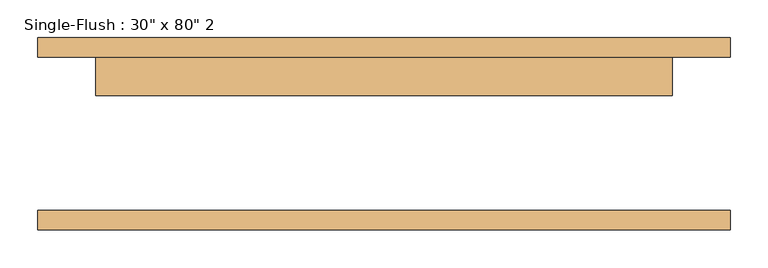
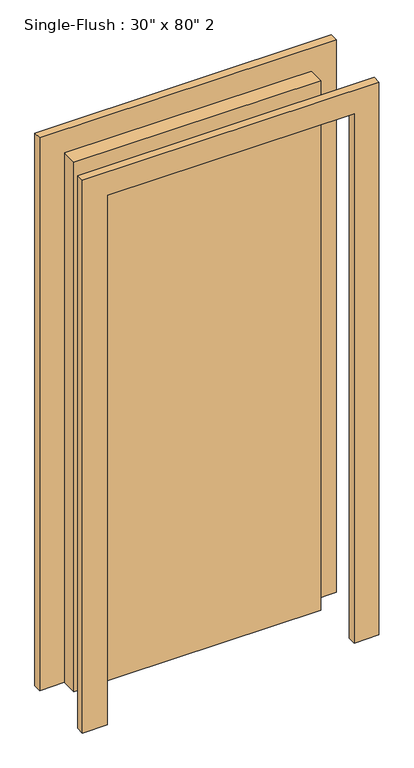
"""IFC4 building model written with IfcOpenShell, lengths in millimetres: door geometry."""

from ifc_helpers import new_model, si_unit, frame, origin, origin_with_axes, place, context, project, spatial, polyline, outline, extrude, source, transform, mapped, element, save


def door_d8ec59b1(model_context):
    return source(origin(), model_context, "Body", "SweptSolid", [
        extrude(outline(polyline([(1803.4, -457.2), (0.0, -457.2), (0.0, -381.0), (1727.2, -381.0), (1727.2, 381.0), (0.0, 381.0), (0.0, 457.2), (1803.4, 457.2), (1803.4, -457.2)])), frame((0.0, 101.6, 0.0), z_axis=(0.0, 1.0, 0.0), x_axis=(0.0, 0.0, 1.0)), (0.0, 0.0, 1.0), 25.4),
        extrude(outline(polyline([(1803.4, 457.2), (1803.4, -457.2), (0.0, -457.2), (0.0, -381.0), (1727.2, -381.0), (1727.2, 381.0), (0.0, 381.0), (0.0, 457.2), (1803.4, 457.2)])), frame((0.0, -127.0, 0.0), z_axis=(0.0, 1.0, 0.0), x_axis=(0.0, 0.0, 1.0)), (0.0, 0.0, 1.0), 25.4),
        extrude(outline(polyline([(381.0, 50.8), (-381.0, 50.8), (-381.0, 101.6), (381.0, 101.6), (381.0, 50.8)])), origin_with_axes(), (0.0, 0.0, 1.0), 1727.2),
    ])


if __name__ == "__main__":
    model = new_model("IFC4")
    model_context = context("Model", 3, world=origin())
    ifc_project = project(units=[si_unit("LENGTHUNIT", "METRE", prefix="MILLI")], contexts=[model_context])
    site = spatial("IfcSite", under=ifc_project)
    building = spatial("IfcBuilding", under=site)
    placement = place(None, origin())
    door_shape = door_d8ec59b1(model_context)
    element("IfcDoor", 1, ObjectType="Single-Flush : 30\" x 80\" 2", at=placement, inside=building, context=model_context, shape_type="MappedRepresentation", body=[
        mapped(door_shape, transform((0.0, 0.0, 0.0), x_axis=(1.0, 0.0, 0.0), y_axis=(0.0, 1.0, 0.0), z_axis=(0.0, 0.0, 1.0))),
    ])
    save(model, "model.ifc")

# Revit data of these elements
# Type "Single-Flush : 30\" x 80\" 2"
#   Type Mark = "9"
#   Construction Type Id = "MDOOR"
#   Assembly Code = "C1020"
#   Analytic Construction = "Metal"
#   Thickness = 0' - 2"
#   Heat Transfer Coefficient (U) = 0.651978 BTU/(h·ft²·°F)
#   Height = 5' - 8"
#   Trim Projection Ext = 0' - 1"
#   Trim Projection Int = 0' - 1"
#   Trim Width = 0' - 3"
#   Width = 2' - 6"
#   Define Thermal Properties by = 1
#   Door Material = Door - Panel
#   Frame Material = Door - Frame
#   Visual Light Transmittance = 0
#   Solar Heat Gain Coefficient = 0
#   Function = (empty or 0)
#   Wall Closure = (empty or 0)
# Element 1 (IfcDoor, "Single-Flush : 30\" x 80\" 2")
#   Materials on its faces: "Door - Frame", "Door - Panel"
# Materials
#   "Door - Panel": class "Wood", colour RGB 210 159 95, transparency 0
#   "Door - Frame": colour RGB 118 70 51, transparency 0
